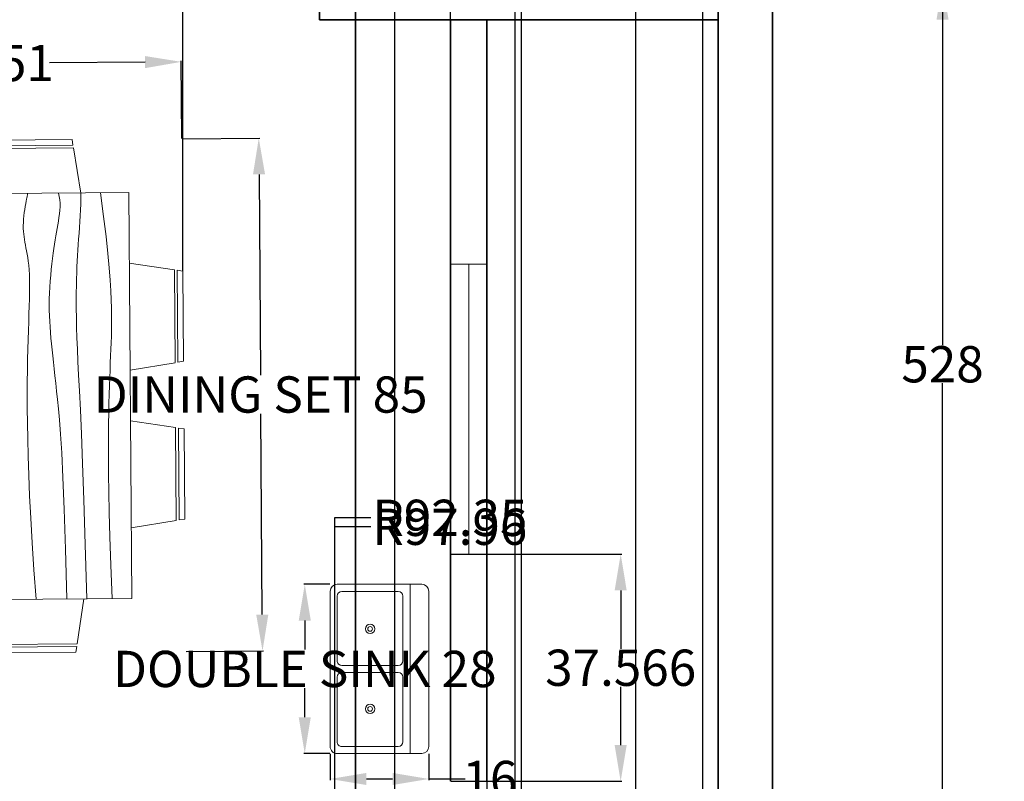
# Model space of a CAD drawing. Units: inches. Extents: x 351 to 774, y 111 to 703.
# Tile 4 of 6: x 608 to 771, y 338 to 464. Entities that reach past the tile are written whole.
import ezdxf

# ---------------------------------------------------------------- set-up
doc = ezdxf.new("R2010")
doc.units = ezdxf.units.IN
doc.header["$MEASUREMENT"] = 0
for name, color, linetype, lineweight in [('A-ANNO-DIMS', 2, 'Continuous', 18), ('A-FLOR-FIXT', 9, 'Continuous', 18), ('A-FURN', 8, 'Continuous', 18), ('A-GLAZ', 4, 'Continuous', 18), ('A-WALL', 7, 'Continuous', 35)]:
    doc.layers.add(name, color=color, linetype=linetype, lineweight=lineweight)
doc.styles.get("Standard").update_dxf_attribs({"font": 'arial.ttf'})
doc.dimstyles.get("Standard").update_dxf_attribs({"dimtxt": 6, "dimasz": 6, "dimexe": 0.18, "dimexo": 0.0625, "dimgap": 0.09, "dimtad": 0, "dimtih": 1, "dimtoh": 1, "dimdec": 0, "dimzin": 0, "dimdsep": 46, "dimlunit": 3, "dimtxsty": 'Standard', "dimcen": 0.09, "dimadec": 0, "dimazin": 0, "dimtfac": 1, "dimtdec": 0, "dimtofl": 0, "dimtmove": 0, "dimatfit": 3, "dimfxl": 1, "dimtolj": 1, "dimtzin": 0, "dimarcsym": 0})

# ---------------------------------------------------------------- blocks, each defined once
blk = doc.blocks.new('Dining Set - 36 x 72 in.')
for p, q in [((-22, 27.5), (-22.1562, 26.50042)), ((-5.8416, 26.5), (-22.1534, 26.5)), ((-22, 27.5), (-6, 27.5)), ((-5.8437, 26.49966), (-6, 27.5)), ((6, 27.5), (5.8438, 26.50042)), ((22.1584, 26.5), (5.8466, 26.5)), ((6, 27.5), (22, 27.5)), ((22.1563, 26.49966), (22, 27.5)), ((-22.2343, 26.00059), (-23.4847, 17.99762)), ((-22.2304, 26), (-5.7608, 26)), ((-4.5152, 17.99762), (-5.7655, 25.99926)), ((5.7657, 26.00059), (4.5153, 17.99762)), ((5.7696, 26), (22.2392, 26)), ((23.4848, 17.99762), (22.2345, 25.99926)), ((36, 18), (-36, 18)), ((-36, 18), (-36, -18)), ((36, -18), (36, 18)), ((-44.0006, 8.23428), (-35.9976, 9.48474)), ((44.0006, 8.23428), (35.9976, 9.48474)), ((-45.5, 8), (-44.5004, 8.15617)), ((-45.5, 8), (-45.5, -8)), ((-44.5, -8.15843), (-44.5, 8.15338)), ((-44, 8.23041), (-44, -8.23915)), ((44, 8.23041), (44, -8.23915)), ((44.5, -8.15843), (44.5, 8.15338)), ((45.5, 8), (44.5005, 8.15617)), ((45.5, 8), (45.5, -8)), ((-44.4997, -8.15631), (-45.5, -8)), ((-35.9976, -9.48476), (-43.9993, -8.2345)), ((35.9976, -9.48476), (43.9993, -8.2345)), ((44.4997, -8.15631), (45.5, -8)), ((-36, -18), (36, -18)), ((-22.2343, -26.0006), (-23.4847, -17.99762)), ((-4.5152, -17.99762), (-5.7655, -25.99928)), ((5.7657, -26.0006), (4.5153, -17.99762)), ((23.4848, -17.99762), (22.2345, -25.99928)), ((-22.2304, -26), (-5.7608, -26)), ((5.7696, -26), (22.2392, -26)), ((-22, -27.5), (-22.1562, -26.50044)), ((-5.8416, -26.5), (-22.1534, -26.5)), ((-22, -27.5), (-6, -27.5)), ((-5.8437, -26.49967), (-6, -27.5)), ((6, -27.5), (5.8438, -26.50044)), ((22.1584, -26.5), (5.8466, -26.5)), ((6, -27.5), (22, -27.5)), ((22.1563, -26.49967), (22, -27.5))]:
    blk.add_line(p, q)
for points in [[(-36, 15), (-31.1772, 14.97754), (-26.8079, 14.91406), (-22.8538, 14.81543), (-19.276, 14.6875), (-16.0362, 14.53613), (-13.0957, 14.36718), (-10.4159, 14.18652), (-7.9583, 14), (-5.6904, 13.81315), (-3.6035, 13.63021), (-1.6954, 13.45508), (0.0365, 13.29166), (1.5945, 13.14388), (2.9811, 13.01562), (4.1988, 12.9108), (5.25, 12.83333), (6.1393, 12.78613), (6.8802, 12.76823), (7.4883, 12.77767), (7.9792, 12.8125), (8.3685, 12.87077), (8.6719, 12.95052), (8.9049, 13.0498), (9.0833, 13.16666), (9.2205, 13.29899), (9.3216, 13.44401), (9.3895, 13.59879), (9.4271, 13.76041), (9.4373, 13.92594), (9.4232, 14.09245), (9.3875, 14.257), (9.3333, 14.41666), (9.2638, 14.56917), (9.1836, 14.71484), (9.0975, 14.85465), (9.0104, 14.98958), (8.9272, 15.1206), (8.8529, 15.2487), (8.7922, 15.37483), (8.75, 15.5), (8.7305, 15.62467), (8.7344, 15.74739), (8.7617, 15.86621), (8.8125, 15.97916), (8.8867, 16.08431), (8.9844, 16.17968), (9.1055, 16.26334), (9.25, 16.33333), (9.4189, 16.38802), (9.6172, 16.42708), (9.8506, 16.45052), (10.125, 16.45833), (10.4463, 16.45052), (10.8203, 16.42708), (11.2529, 16.38802), (11.75, 16.33333), (12.3184, 16.26318), (12.9694, 16.17838), (13.7151, 16.07991), (14.5677, 15.96875), (15.5395, 15.84586), (16.6426, 15.71224), (17.8893, 15.56884), (19.2917, 15.41666), (20.859, 15.25667), (22.5879, 15.08984), (24.4721, 14.91715), (26.5052, 14.73958), (28.6809, 14.5581), (30.9929, 14.3737), (33.4347, 14.18733), (36, 14)], [(-36, 10), (-28.9766, 10.14274), (-23.1725, 10.20442), (-18.4241, 10.19775), (-14.5677, 10.13541), (-11.4399, 10.03011), (-8.877, 9.89453), (-6.7154, 9.74137), (-4.7917, 9.58333), (-2.9698, 9.43082), (-1.2246, 9.28515), (0.4415, 9.14534), (2.026, 9.01041), (3.5266, 8.87939), (4.9408, 8.7513), (6.266, 8.62516), (7.5, 8.5), (8.6411, 8.37549), (9.6914, 8.2539), (10.6538, 8.13818), (11.5312, 8.03125), (12.3267, 7.93603), (13.043, 7.85547), (13.6831, 7.79248), (14.25, 7.75), (14.7471, 7.7303), (15.1797, 7.73307), (15.5537, 7.75732), (15.875, 7.80208), (16.1494, 7.86637), (16.3828, 7.94922), (16.5811, 8.04964), (16.75, 8.16666), (16.8944, 8.29915), (17.0143, 8.44531), (17.1089, 8.60319), (17.1771, 8.77083), (17.218, 8.94629), (17.2305, 9.1276), (17.2137, 9.31282), (17.1667, 9.5), (17.0895, 9.6875), (16.987, 9.875), (16.8649, 10.0625), (16.7292, 10.25), (16.5856, 10.4375), (16.4401, 10.625), (16.2985, 10.8125), (16.1667, 11), (16.05, 11.18733), (15.9518, 11.3737), (15.8752, 11.5581), (15.8229, 11.73958), (15.798, 11.91715), (15.8034, 12.08984), (15.842, 12.25667), (15.9167, 12.41666), (16.0295, 12.56836), (16.1784, 12.70833), (16.3605, 12.83268), (16.5729, 12.9375), (16.8127, 13.01888), (17.0768, 13.07291), (17.3625, 13.0957), (17.6667, 13.08333), (17.9894, 13.03312), (18.3418, 12.94726), (18.7382, 12.82918), (19.1927, 12.68229), (19.7195, 12.51001), (20.3327, 12.31575), (21.0465, 12.10294), (21.875, 11.875), (22.8357, 11.63354), (23.959, 11.37304), (25.2786, 11.08618), (26.8282, 10.76562), (28.6414, 10.40405), (30.752, 9.99414), (33.1936, 9.52856), (36, 9)], [(-36, 5.5), (-30.7157, 5.3348), (-26.069, 5.20963), (-21.9946, 5.11767), (-18.4271, 5.05208), (-15.3009, 5.00602), (-12.5508, 4.97265), (-10.1112, 4.94515), (-7.9167, 4.91666), (-5.909, 4.88167), (-4.0586, 4.83984), (-2.3429, 4.79215), (-0.7396, 4.73958), (0.7739, 4.6831), (2.22, 4.6237), (3.6213, 4.56233), (5, 4.5), (6.373, 4.43782), (7.7344, 4.3776), (9.0723, 4.32129), (10.375, 4.27083), (11.6309, 4.22819), (12.8281, 4.19531), (13.9551, 4.17415), (15, 4.16666), (15.954, 4.17448), (16.819, 4.19791), (17.6001, 4.23698), (18.3021, 4.29166), (18.9299, 4.36198), (19.4883, 4.44791), (19.9823, 4.54948), (20.4167, 4.66666), (20.7969, 4.79899), (21.1302, 4.94401), (21.4245, 5.09879), (21.6875, 5.26041), (21.9271, 5.42594), (22.1511, 5.59245), (22.3672, 5.757), (22.5834, 5.91666), (22.8065, 6.06868), (23.0404, 6.21093), (23.2879, 6.34147), (23.5521, 6.45833), (23.8358, 6.55957), (24.142, 6.64323), (24.4735, 6.70735), (24.8334, 6.75), (25.2235, 6.76969), (25.642, 6.76692), (26.0858, 6.74267), (26.5521, 6.69791), (27.0379, 6.63362), (27.5404, 6.55078), (28.0565, 6.45036), (28.5834, 6.33333), (29.1242, 6.19987), (29.7071, 6.04687), (30.3661, 5.87044), (31.1354, 5.66666), (32.0493, 5.43164), (33.142, 5.16146), (34.4475, 4.85221), (36, 4.5)], [(-36, -1), (-30.7915, -0.6591), (-26.0195, -0.38216), (-21.6519, -0.16284), (-17.6563, 0.00521), (-14.0005, 0.12833), (-10.6523, 0.21289), (-7.5796, 0.26522), (-4.75, 0.29166), (-2.134, 0.29793), (0.2878, 0.28711), (2.5317, 0.26163), (4.6146, 0.22396), (6.5529, 0.17651), (8.3633, 0.12174), (10.0623, 0.06209), (11.6667, 0), (13.1899, -0.06201), (14.6341, -0.1211), (15.9982, -0.17432), (17.2813, -0.21875), (18.4823, -0.25147), (19.6003, -0.26953), (20.6343, -0.27002), (21.5834, -0.25), (22.4481, -0.20768), (23.2357, -0.14584), (23.9549, -0.06836), (24.6146, 0.02083), (25.2235, 0.11784), (25.7904, 0.21875), (26.3241, 0.31966), (26.8334, 0.41666), (27.3265, 0.50618), (27.8099, 0.58593), (28.2894, 0.65397), (28.7709, 0.70833), (29.2601, 0.74707), (29.763, 0.76823), (30.2855, 0.76985), (30.8334, 0.75), (31.4088, 0.70784), (31.9994, 0.64713), (32.589, 0.57275), (33.1615, 0.48958), (33.7008, 0.4025), (34.1908, 0.3164), (34.6153, 0.23616), (34.9584, 0.16666), (35.2099, 0.11165), (35.3848, 0.07031), (35.504, 0.04069), (35.5886, 0.02083), (35.6594, 0.00879), (35.7377, 0.0026), (35.8442, 0.00032), (36, 0)], [(-36, -6.5), (-27.1843, -6.31267), (-20.084, -6.1263), (-14.469, -5.9419), (-10.1094, -5.76042), (-6.7752, -5.58285), (-4.2363, -5.41016), (-2.2629, -5.24333), (-0.625, -5.08334), (0.8708, -4.93099), (2.2715, -4.78646), (3.5872, -4.64974), (4.8281, -4.52084), (6.0046, -4.39974), (7.127, -4.28646), (8.2053, -4.18099), (9.25, -4.08334), (10.2705, -3.99382), (11.2734, -3.91407), (12.2647, -3.84603), (13.25, -3.79167), (14.2354, -3.75293), (15.2266, -3.73177), (16.2295, -3.73015), (17.25, -3.75), (18.2912, -3.79248), (19.3451, -3.85547), (20.4009, -3.93604), (21.4479, -4.03125), (22.4754, -4.13819), (23.4727, -4.25391), (24.4289, -4.37549), (25.3334, -4.5), (26.1785, -4.62492), (26.9694, -4.74935), (27.7145, -4.87281), (28.4219, -4.99479), (29.1, -5.11483), (29.7572, -5.23242), (30.4016, -5.34709), (31.0417, -5.45834), (31.6837, -5.56437), (32.3262, -5.65821), (32.9658, -5.73153), (33.599, -5.77604), (34.2224, -5.78345), (34.8327, -5.74545), (35.4264, -5.65373), (36, -5.5)], [(-36, -10), (-26.4022, -9.81299), (-18.4675, -9.62891), (-11.9839, -9.45069), (-6.7396, -9.28125), (-2.5226, -9.12354), (0.8789, -8.98047), (3.6769, -8.85498), (6.0833, -8.75), (8.2767, -8.66765), (10.3021, -8.60677), (12.1712, -8.56543), (13.8958, -8.54167), (15.4876, -8.53353), (16.9583, -8.53907), (18.3197, -8.55632), (19.5834, -8.58334), (20.7616, -8.61841), (21.8685, -8.66081), (22.9188, -8.71004), (23.9271, -8.76563), (24.9081, -8.82707), (25.8763, -8.89388), (26.8465, -8.96558), (27.8334, -9.04167), (28.8474, -9.12118), (29.8828, -9.20117), (30.93, -9.27824), (31.9792, -9.34896), (33.0205, -9.40991), (34.0443, -9.45768), (35.0407, -9.48885), (36, -9.5)], [(-36, -14.5), (-30.0881, -14.33513), (-25.0332, -14.21224), (-20.7312, -14.12647), (-17.0781, -14.07292), (-13.97, -14.04671), (-11.3027, -14.04297), (-8.9724, -14.05681), (-6.875, -14.08334), (-4.9224, -14.11833), (-3.0905, -14.16016), (-1.3709, -14.20785), (0.2448, -14.26042), (1.7647, -14.3169), (3.1973, -14.3763), (4.5507, -14.43767), (5.8333, -14.5), (7.0554, -14.5621), (8.235, -14.62175), (9.3922, -14.67652), (10.5469, -14.72396), (11.7192, -14.76164), (12.929, -14.78711), (14.1965, -14.79794), (15.5417, -14.79167), (16.9933, -14.76424), (18.6152, -14.70508), (20.4804, -14.60197), (22.6615, -14.44271), (25.2312, -14.21509), (28.2624, -13.9069), (31.8277, -13.50594), (36, -13)]]:
    blk.add_lwpolyline(points)
blk = doc.blocks.new('Sink-double - 36 in top')
for p, q in [((-18, -4), (18, -4)), ((-0.75, -18.5), (-0.75, -6.5)), ((0.75, -6.5), (0.75, -18.5))]:
    blk.add_line(p, q)
for points in [[(-16.5, 0), (16.5, 0)], [(-18, -19.5), (-18, -1.5)], [(18, -1.5), (18, -19.5)], [(-15.5, -5.5), (-1.75, -5.5)], [(1.75, -5.5), (15.5, -5.5)], [(-16.5, -18.5), (-16.5, -6.5)], [(16.5, -6.5), (16.5, -18.5)], [(-1.75, -19.5), (-15.5, -19.5)], [(15.5, -19.5), (1.75, -19.5)], [(16.5, -21), (-16.5, -21)]]:
    blk.add_lwpolyline(points)
for centre, radius in [((-8.5, -12.5), 1), ((-8.5, -12.5), 0.5), ((8.5, -12.5), 1), ((8.5, -12.5), 0.5)]:
    blk.add_circle(centre, radius)
for centre, radius, start, end in [((-16.5, -1.5), 1.5, 90, 180), ((16.5, -1.5), 1.5, 0, 90), ((-15.5, -6.5), 1, 90, 180), ((-1.75, -6.5), 1, 0, 90), ((1.75, -6.5), 1, 90, 180), ((15.5, -6.5), 1, 0, 90), ((-15.5, -18.5), 1, 180, 270), ((-1.75, -18.5), 1, 270, 0), ((1.75, -18.5), 1, 180, 270), ((15.5, -18.5), 1, 270, 0), ((-16.5, -19.5), 1.5, 180, 270), ((16.5, -19.5), 1.5, 270, 0)]:
    blk.add_arc(centre, radius, start, end)
blk = doc.blocks.new('WIN-48IN-6IN-WALL')
blk.add_line((3, 48), (3, 0))
blk.add_lwpolyline([(0, 48), (6, 48), (6, 0), (0, 0)], close=True)
blk = doc.blocks.new('*D32')
at = {"layer": 'A-ANNO-DIMS', "color": 0, "lineweight": -2, "transparency": 16777216}
for p, q in [((696.79, 480.27), (696.79, 476.4)), ((721.84, 480.27), (721.84, 476.4)), ((702.79, 476.58), (715.84, 476.58)), ((721.84, 476.58), (727.84, 476.58))]:
    blk.add_line(p, q, dxfattribs=at)
at = {"layer": 'A-ANNO-DIMS', "color": 0, "transparency": 16777216}
for points in [[(702.79, 477.58), (702.79, 475.58), (696.79, 476.58)], [(715.84, 477.58), (715.84, 475.58), (721.84, 476.58)]]:
    blk.add_solid(points, dxfattribs=at)
at = {"layer": 'Defpoints', "color": 0, "transparency": 16777216}
for p in [(696.79, 480.33), (721.84, 480.33), (721.84, 476.58)]:
    blk.add_point(p, dxfattribs=at)
at = {"layer": 'A-ANNO-DIMS', "color": 0, "transparency": 16777216, "insert": (750.8, 476.58), "char_height": 6, "attachment_point": 5}
blk.add_mtext('\\A1;WC 25 TYP.', dxfattribs=at)
blk = doc.blocks.new('*D36')
at = {"layer": 'A-ANNO-DIMS', "color": 0, "lineweight": -2, "transparency": 16777216}
for p, q in [((635.35, 444.55), (648.2, 444.64)), ((648.06, 438.64), (648.31, 405.42)), ((648.6, 365.81), (648.35, 399.03)), ((635.98, 359.72), (648.82, 359.81))]:
    blk.add_line(p, q, dxfattribs=at)
at = {"layer": 'A-ANNO-DIMS', "color": 0, "transparency": 16777216}
for points in [[(649.06, 438.65), (647.06, 438.64), (648.02, 444.64)], [(649.6, 365.82), (647.6, 365.8), (648.64, 359.81)]]:
    blk.add_solid(points, dxfattribs=at)
at = {"layer": 'Defpoints', "color": 0, "transparency": 16777216}
for p in [(635.29, 444.55), (648.02, 444.64), (635.92, 359.72)]:
    blk.add_point(p, dxfattribs=at)
at = {"layer": 'A-ANNO-DIMS', "color": 0, "transparency": 16777216, "insert": (648.33, 402.23), "char_height": 6, "attachment_point": 5}
blk.add_mtext('\\A1;DINING SET 85', dxfattribs=at)
blk = doc.blocks.new('*D37')
at = {"layer": 'A-ANNO-DIMS', "color": 0, "lineweight": -2, "transparency": 16777216}
for p, q in [((584.02, 444.23), (583.93, 457.08)), ((589.93, 456.94), (605.75, 457.06)), ((629.2, 457.23), (613.37, 457.11)), ((635.29, 444.61), (635.2, 457.45))]:
    blk.add_line(p, q, dxfattribs=at)
at = {"layer": 'A-ANNO-DIMS', "color": 0, "transparency": 16777216}
for points in [[(629.19, 458.23), (629.21, 456.23), (635.2, 457.27)], [(589.92, 457.94), (589.93, 455.94), (583.93, 456.9)]]:
    blk.add_solid(points, dxfattribs=at)
at = {"layer": 'Defpoints', "color": 0, "transparency": 16777216}
for p in [(583.93, 456.9), (584.02, 444.17), (635.29, 444.55)]:
    blk.add_point(p, dxfattribs=at)
at = {"layer": 'A-ANNO-DIMS', "color": 0, "transparency": 16777216, "insert": (609.56, 457.08), "char_height": 6, "attachment_point": 5}
blk.add_mtext('\\A1;51', dxfattribs=at)
blk = doc.blocks.new('*D38')
at = {"layer": 'A-ANNO-DIMS', "color": 0, "lineweight": -2, "transparency": 16777216}
for p, q in [((659.77, 370.83), (655.45, 370.83)), ((655.63, 364.83), (655.63, 360.03)), ((655.63, 348.83), (655.63, 353.64)), ((659.77, 342.83), (655.45, 342.83))]:
    blk.add_line(p, q, dxfattribs=at)
at = {"layer": 'A-ANNO-DIMS', "color": 0, "transparency": 16777216}
for points in [[(654.63, 364.83), (656.63, 364.83), (655.63, 370.83)], [(654.63, 348.83), (656.63, 348.83), (655.63, 342.83)]]:
    blk.add_solid(points, dxfattribs=at)
at = {"layer": 'Defpoints', "color": 0, "transparency": 16777216}
for p in [(659.83, 370.83), (655.63, 342.83), (659.83, 342.83)]:
    blk.add_point(p, dxfattribs=at)
at = {"layer": 'A-ANNO-DIMS', "color": 0, "transparency": 16777216, "insert": (655.63, 356.83), "char_height": 6, "attachment_point": 5}
blk.add_mtext('\\A1;DOUBLE SINK 28', dxfattribs=at)
blk = doc.blocks.new('*D39')
at = {"layer": 'A-ANNO-DIMS', "color": 0, "lineweight": -2, "transparency": 16777216}
for p, q in [((659.83, 342.77), (659.83, 338.45)), ((676.17, 342.77), (676.17, 338.45)), ((665.83, 338.63), (670.17, 338.63)), ((676.17, 338.63), (682.17, 338.63))]:
    blk.add_line(p, q, dxfattribs=at)
at = {"layer": 'A-ANNO-DIMS', "color": 0, "transparency": 16777216}
for points in [[(665.83, 339.63), (665.83, 337.63), (659.83, 338.63)], [(670.17, 339.63), (670.17, 337.63), (676.17, 338.63)]]:
    blk.add_solid(points, dxfattribs=at)
at = {"layer": 'Defpoints', "color": 0, "transparency": 16777216}
for p in [(659.83, 342.83), (676.17, 342.83), (676.17, 338.63)]:
    blk.add_point(p, dxfattribs=at)
at = {"layer": 'A-ANNO-DIMS', "color": 0, "transparency": 16777216, "insert": (686.27, 338.63), "char_height": 6, "attachment_point": 5}
blk.add_mtext('\\A1;16', dxfattribs=at)
blk = doc.blocks.new('*D47')
at = {"layer": 'A-ANNO-DIMS', "color": 0, "lineweight": -2, "transparency": 16777216}
for p, q in [((733.11, 671.24), (761.37, 671.24)), ((761.19, 665.24), (761.19, 410.4)), ((761.19, 149.24), (761.19, 404.09)), ((733.11, 143.24), (761.37, 143.24))]:
    blk.add_line(p, q, dxfattribs=at)
at = {"layer": 'A-ANNO-DIMS', "color": 0, "transparency": 16777216}
for points in [[(760.19, 665.24), (762.19, 665.24), (761.19, 671.24)], [(760.19, 149.24), (762.19, 149.24), (761.19, 143.24)]]:
    blk.add_solid(points, dxfattribs=at)
at = {"layer": 'Defpoints', "color": 0, "transparency": 16777216}
for p in [(733.04, 671.24), (761.19, 671.24), (733.04, 143.24)]:
    blk.add_point(p, dxfattribs=at)
at = {"layer": 'A-ANNO-DIMS', "color": 0, "transparency": 16777216, "insert": (761.19, 407.24), "char_height": 6, "attachment_point": 5}
blk.add_mtext('\\A1;528', dxfattribs=at)
blk = doc.blocks.new('*D68')
at = {"layer": 'A-ANNO-DIMS', "color": 0, "lineweight": -2, "transparency": 16777216}
for p, q in [((685.77, 338.18), (685.77, 114.91)), ((724.04, 338.18), (724.04, 114.91)), ((691.77, 115.09), (694.69, 115.09)), ((718.04, 115.09), (715.12, 115.09))]:
    blk.add_line(p, q, dxfattribs=at)
at = {"layer": 'A-ANNO-DIMS', "color": 0, "transparency": 16777216}
for points in [[(691.77, 116.09), (691.77, 114.09), (685.77, 115.09)], [(718.04, 116.09), (718.04, 114.09), (724.04, 115.09)]]:
    blk.add_solid(points, dxfattribs=at)
at = {"layer": 'Defpoints', "color": 0, "transparency": 16777216}
for p in [(685.77, 338.24), (724.04, 338.24), (724.04, 115.09)]:
    blk.add_point(p, dxfattribs=at)
at = {"layer": 'A-ANNO-DIMS', "color": 0, "transparency": 16777216, "insert": (704.9, 115.09), "char_height": 6, "attachment_point": 5}
blk.add_mtext('\\A1;38.28', dxfattribs=at)
blk = doc.blocks.new('*D69')
at = {"layer": 'A-ANNO-DIMS', "color": 0, "lineweight": -2, "transparency": 16777216}
for p, q in [((724.04, 473.44), (724.04, 114.91)), ((664.04, 470.18), (664.04, 114.91)), ((670.04, 115.09), (689.65, 115.09)), ((718.04, 115.09), (698.44, 115.09))]:
    blk.add_line(p, q, dxfattribs=at)
at = {"layer": 'A-ANNO-DIMS', "color": 0, "transparency": 16777216}
for points in [[(670.04, 116.09), (670.04, 114.09), (664.04, 115.09)], [(718.04, 116.09), (718.04, 114.09), (724.04, 115.09)]]:
    blk.add_solid(points, dxfattribs=at)
at = {"layer": 'Defpoints', "color": 0, "transparency": 16777216}
for p in [(724.04, 473.5), (664.04, 470.24), (724.04, 115.09)]:
    blk.add_point(p, dxfattribs=at)
at = {"layer": 'A-ANNO-DIMS', "color": 0, "transparency": 16777216, "insert": (694.04, 115.09), "char_height": 6, "attachment_point": 5}
blk.add_mtext('\\A1;60', dxfattribs=at)
blk = doc.blocks.new('*D81')
at = {"layer": 'A-ANNO-DIMS', "color": 0, "lineweight": -2, "transparency": 16777216}
for p, q in [((679.83, 375.81), (708.1, 375.81)), ((707.92, 369.81), (707.92, 360.18)), ((707.92, 344.24), (707.92, 353.87)), ((679.83, 338.24), (708.1, 338.24))]:
    blk.add_line(p, q, dxfattribs=at)
at = {"layer": 'A-ANNO-DIMS', "color": 0, "transparency": 16777216}
for points in [[(706.92, 369.81), (708.92, 369.81), (707.92, 375.81)], [(706.92, 344.24), (708.92, 344.24), (707.92, 338.24)]]:
    blk.add_solid(points, dxfattribs=at)
at = {"layer": 'Defpoints', "color": 0, "transparency": 16777216}
for p in [(679.77, 375.81), (679.77, 338.24), (707.92, 338.24)]:
    blk.add_point(p, dxfattribs=at)
at = {"layer": 'A-ANNO-DIMS', "color": 0, "transparency": 16777216, "insert": (707.92, 357.03), "char_height": 6, "attachment_point": 5}
blk.add_mtext('\\A1;37.566', dxfattribs=at)
blk = doc.blocks.new('*D86')
at = {"layer": 'A-ANNO-DIMS', "color": 0, "lineweight": -2, "transparency": 16777216}
for p, q in [((710.41, 152.3), (710.41, 699.57)), ((716.41, 699.39), (718.04, 699.39)), ((724.04, 152.3), (724.04, 699.57)), ((724.04, 699.39), (730.04, 699.39))]:
    blk.add_line(p, q, dxfattribs=at)
at = {"layer": 'A-ANNO-DIMS', "color": 0, "transparency": 16777216}
for points in [[(716.41, 700.39), (716.41, 698.39), (710.41, 699.39)], [(718.04, 700.39), (718.04, 698.39), (724.04, 699.39)]]:
    blk.add_solid(points, dxfattribs=at)
at = {"layer": 'Defpoints', "color": 0, "transparency": 16777216}
for p in [(724.04, 699.39), (710.41, 152.24), (724.04, 152.24)]:
    blk.add_point(p, dxfattribs=at)
at = {"layer": 'A-ANNO-DIMS', "color": 0, "transparency": 16777216, "insert": (742.3, 699.39), "char_height": 6, "attachment_point": 5}
blk.add_mtext('\\A1;13.633', dxfattribs=at)
blk = doc.blocks.new('*D87')
at = {"layer": 'A-ANNO-DIMS', "color": 0, "lineweight": -2, "transparency": 16777216}
for p, q in [((691.51, 206.3), (691.51, 699.57)), ((697.51, 699.39), (702.14, 699.39)), ((715.51, 699.39), (710.89, 699.39)), ((721.51, 206.3), (721.51, 699.57))]:
    blk.add_line(p, q, dxfattribs=at)
at = {"layer": 'A-ANNO-DIMS', "color": 0, "transparency": 16777216}
for points in [[(697.51, 700.39), (697.51, 698.39), (691.51, 699.39)], [(715.51, 700.39), (715.51, 698.39), (721.51, 699.39)]]:
    blk.add_solid(points, dxfattribs=at)
at = {"layer": 'Defpoints', "color": 0, "transparency": 16777216}
for p in [(721.51, 699.39), (691.51, 206.24), (721.51, 206.24)]:
    blk.add_point(p, dxfattribs=at)
at = {"layer": 'A-ANNO-DIMS', "color": 0, "transparency": 16777216, "insert": (706.51, 699.39), "char_height": 6, "attachment_point": 5}
blk.add_mtext('\\A1;30', dxfattribs=at)
blk = doc.blocks.new('*D88')
at = {"layer": 'A-ANNO-DIMS', "color": 0, "lineweight": -2, "transparency": 16777216}
for p, q in [((658.043027, 699.392076), (652.043027, 699.392076)), ((664.043027, 200.304576), (664.043027, 699.572076)), ((691.510725, 200.304576), (691.510725, 699.572076)), ((697.510725, 699.392076), (703.510725, 699.392076))]:
    blk.add_line(p, q, dxfattribs=at)
at = {"layer": 'A-ANNO-DIMS', "color": 0, "transparency": 16777216}
for points in [[(658.043027, 700.392076), (658.043027, 698.392076), (664.043027, 699.392076)], [(697.510725, 700.392076), (697.510725, 698.392076), (691.510725, 699.392076)]]:
    blk.add_solid(points, dxfattribs=at)
at = {"layer": 'Defpoints', "color": 0, "transparency": 16777216}
for p in [(691.510725, 699.392076), (664.043027, 200.242076), (691.510725, 200.242076)]:
    blk.add_point(p, dxfattribs=at)
at = {"layer": 'A-ANNO-DIMS', "color": 0, "transparency": 16777216, "insert": (677.776876, 699.392076), "char_height": 6, "attachment_point": 5}
blk.add_mtext('\\A1;27.47', dxfattribs=at)
blk = doc.blocks.new('*D96')
at = {"layer": 'A-ANNO-DIMS', "color": 0, "lineweight": -2, "transparency": 16777216}
for p, q in [((635.45, 422.7), (635.45, 699.57)), ((641.45, 699.39), (647.85, 699.39)), ((673.77, 699.39), (667.36, 699.39)), ((679.77, 423.87), (679.77, 699.57))]:
    blk.add_line(p, q, dxfattribs=at)
at = {"layer": 'A-ANNO-DIMS', "color": 0, "transparency": 16777216}
for points in [[(641.45, 700.39), (641.45, 698.39), (635.45, 699.39)], [(673.77, 700.39), (673.77, 698.39), (679.77, 699.39)]]:
    blk.add_solid(points, dxfattribs=at)
at = {"layer": 'Defpoints', "color": 0, "transparency": 16777216}
for p in [(679.77, 699.39), (679.77, 423.81), (635.45, 422.64)]:
    blk.add_point(p, dxfattribs=at)
at = {"layer": 'A-ANNO-DIMS', "color": 0, "transparency": 16777216, "insert": (657.61, 699.39), "char_height": 6, "attachment_point": 5}
blk.add_mtext('\\A1;44.31', dxfattribs=at)
blk = doc.blocks.new('*D101')
at = {"layer": 'A-ANNO-DIMS', "color": 0, "lineweight": -2, "transparency": 16777216}
for p, q in [((658.04, 699.39), (652.04, 699.39)), ((664.04, 152.3), (664.04, 699.57)), ((690.48, 153.55), (690.48, 699.57)), ((696.48, 699.39), (702.48, 699.39))]:
    blk.add_line(p, q, dxfattribs=at)
at = {"layer": 'A-ANNO-DIMS', "color": 0, "transparency": 16777216}
for points in [[(658.04, 700.39), (658.04, 698.39), (664.04, 699.39)], [(696.48, 700.39), (696.48, 698.39), (690.48, 699.39)]]:
    blk.add_solid(points, dxfattribs=at)
at = {"layer": 'Defpoints', "color": 0, "transparency": 16777216}
for p in [(664.04, 699.39), (690.48, 153.49), (664.04, 152.24)]:
    blk.add_point(p, dxfattribs=at)
at = {"layer": 'A-ANNO-DIMS', "color": 0, "transparency": 16777216, "insert": (677.26, 699.39), "char_height": 6, "attachment_point": 5}
blk.add_mtext('\\A1;26.433', dxfattribs=at)
blk = doc.blocks.new('*D103')
at = {"layer": 'A-ANNO-DIMS', "color": 0, "lineweight": -2, "transparency": 16777216}
for p, q in [((761.19, 486.33), (761.19, 492.33)), ((721.9, 480.33), (761.37, 480.33)), ((724.11, 470.24), (761.37, 470.24)), ((761.19, 464.24), (761.19, 458.24))]:
    blk.add_line(p, q, dxfattribs=at)
at = {"layer": 'A-ANNO-DIMS', "color": 0, "transparency": 16777216}
for points in [[(760.19, 486.33), (762.19, 486.33), (761.19, 480.33)], [(760.19, 464.24), (762.19, 464.24), (761.19, 470.24)]]:
    blk.add_solid(points, dxfattribs=at)
at = {"layer": 'Defpoints', "color": 0, "transparency": 16777216}
for p in [(721.84, 480.33), (724.04, 470.24), (761.19, 470.24)]:
    blk.add_point(p, dxfattribs=at)
at = {"layer": 'A-ANNO-DIMS', "color": 0, "transparency": 16777216, "insert": (761.19, 475.29), "char_height": 6, "attachment_point": 5}
blk.add_mtext('\\A1;10.09', dxfattribs=at)
blk = doc.blocks.new('*D108')
at = {"layer": 'A-ANNO-DIMS', "color": 0, "lineweight": -2, "transparency": 16777216}
for p, q in [((664.04, 527.44), (664.04, 114.91)), ((670.51, 515.76), (670.51, 114.91)), ((658.04, 115.09), (652.04, 115.09)), ((676.51, 115.09), (682.51, 115.09))]:
    blk.add_line(p, q, dxfattribs=at)
at = {"layer": 'A-ANNO-DIMS', "color": 0, "transparency": 16777216}
for points in [[(658.04, 116.09), (658.04, 114.09), (664.04, 115.09)], [(676.51, 116.09), (676.51, 114.09), (670.51, 115.09)]]:
    blk.add_solid(points, dxfattribs=at)
at = {"layer": 'Defpoints', "color": 0, "transparency": 16777216}
for p in [(664.04, 527.5), (670.51, 515.82), (664.04, 115.09)]:
    blk.add_point(p, dxfattribs=at)
at = {"layer": 'A-ANNO-DIMS', "color": 0, "transparency": 16777216, "insert": (641.84, 115.09), "char_height": 6, "attachment_point": 5}
blk.add_mtext('\\A1;6.472', dxfattribs=at)
blk = doc.blocks.new('*D110')
at = {"layer": 'A-ANNO-DIMS', "color": 0, "lineweight": -2, "transparency": 16777216}
for p, q in [((666.56, 380.35), (660.56, 380.35)), ((660.56, 380.35), (660.56, 327.58)), ((660.47, 223.61), (660.65, 223.61)), ((660.56, 223.52), (660.56, 223.7))]:
    blk.add_line(p, q, dxfattribs=at)
at = {"layer": 'A-ANNO-DIMS', "color": 0, "transparency": 16777216}
blk.add_solid([(659.56, 327.58), (661.56, 327.58), (660.56, 321.58)], dxfattribs=at)
at = {"layer": 'Defpoints', "color": 0, "transparency": 16777216}
for p in [(660.56, 321.58), (660.56, 223.61)]:
    blk.add_point(p, dxfattribs=at)
at = {"layer": 'A-ANNO-DIMS', "color": 0, "transparency": 16777216, "insert": (679.64, 380.35), "char_height": 6, "attachment_point": 5}
blk.add_mtext('\\A1;R97.96', dxfattribs=at)
blk = doc.blocks.new('*D111')
at = {"layer": 'A-ANNO-DIMS', "color": 0, "lineweight": -2, "transparency": 16777216}
for p, q in [((666.56, 381.83), (660.56, 381.83)), ((660.56, 381.83), (660.56, 332.43)), ((660.47, 234.08), (660.65, 234.08)), ((660.56, 233.99), (660.56, 234.17))]:
    blk.add_line(p, q, dxfattribs=at)
at = {"layer": 'A-ANNO-DIMS', "color": 0, "transparency": 16777216}
blk.add_solid([(659.56, 332.43), (661.56, 332.43), (660.56, 326.43)], dxfattribs=at)
at = {"layer": 'Defpoints', "color": 0, "transparency": 16777216}
for p in [(660.56, 326.43), (660.56, 234.08)]:
    blk.add_point(p, dxfattribs=at)
at = {"layer": 'A-ANNO-DIMS', "color": 0, "transparency": 16777216, "insert": (679.66, 381.83), "char_height": 6, "attachment_point": 5}
blk.add_mtext('\\A1;R92.35', dxfattribs=at)

msp = doc.modelspace()

# ---------------------------------------------------------------- linework, layer by layer
at = {"layer": 'A-WALL'}
for p, q in [((658.043, 470.2421), (658.043, 464.2421)), ((658.043, 464.2421), (724.043, 464.2421)), ((679.7664, 464.2421), (679.7664, 338.2421)), ((685.7664, 464.2421), (685.7664, 338.2421)), ((724.043, 464.2421), (724.043, 338.2421))]:
    msp.add_line(p, q, dxfattribs=at)
msp.add_lwpolyline([(436.7781, 143.2421), (421.043, 143.2421), (421.043, 671.2421), (733.043, 671.2421), (733.043, 143.2421), (562.043, 143.2421)], dxfattribs=at)

# ---------------------------------------------------------------- block references
at = {"layer": 'A-FLOR-FIXT', "xscale": 0.7777777777777778, "yscale": 0.7777777777777778, "zscale": 0.7777777777777778, "rotation": 270}
msp.add_blockref('Sink-double - 36 in top', (676.1667, 356.8333), dxfattribs=at)
at = {"layer": 'A-FURN', "xscale": 0.9322251862135446, "yscale": 0.9322251862135446, "zscale": 0.9322251862135446, "rotation": 90.42208138352696}
msp.add_blockref('Dining Set - 36 x 72 in.', (609.9687, 401.9447), dxfattribs=at)
at = {"layer": 'A-GLAZ'}
msp.add_blockref('WIN-48IN-6IN-WALL', (679.7664, 375.8083), dxfattribs=at)

# ---------------------------------------------------------------- dimensions: what is measured, and where the dimension line sits
at = {"layer": 'A-ANNO-DIMS'}
for base, p1, p2, override, picture, middle in [((679.7664, 699.3921), (635.4531, 422.6419), (679.7664, 423.8083), {"dimdec": 2, "dimlfac": 1, "dimrnd": 0, "dimzin": 0, "dimdsep": 46, "dimlunit": 2}, '*D96', (657.6098, 699.3921)), ((691.5107, 699.3921), (664.043, 200.2421), (691.5107, 200.2421), {"dimdec": 2, "dimlfac": 1, "dimrnd": 0, "dimzin": 0, "dimdsep": 46, "dimlunit": 2}, '*D88', (677.7769, 699.3921)), ((664.043, 699.3921), (690.4757, 153.4918), (664.043, 152.2421), {"dimdec": 3, "dimlfac": 1, "dimrnd": 0, "dimzin": 0, "dimdsep": 46, "dimlunit": 2}, '*D101', (677.2594, 699.3921)), ((721.5107, 699.3921), (691.5107, 206.2421), (721.5107, 206.2421), {"dimdec": 0, "dimlfac": 1, "dimrnd": 0, "dimzin": 0, "dimdsep": 46, "dimlunit": 2}, '*D87', (706.5107, 699.3921)), ((724.043, 699.3921), (710.4102, 152.2421), (724.043, 152.2421), {"dimdec": 3, "dimlfac": 1, "dimrnd": 0, "dimzin": 0, "dimdsep": 46, "dimlunit": 2}, '*D86', (742.3049, 699.3921)), ((664.043, 115.0921), (670.5147, 515.8184), (664.043, 527.5), {"dimdec": 3, "dimlfac": 1, "dimrnd": 0, "dimzin": 0, "dimdsep": 46, "dimlunit": 2}, '*D108', (641.8439, 115.0921)), ((724.043, 115.0921), (664.043, 470.2421), (724.043, 473.5), {"dimdec": 0, "dimlfac": 1, "dimrnd": 0, "dimzin": 0, "dimdsep": 46, "dimlunit": 2}, '*D69', (694.043, 115.0921)), ((676.1667, 338.6333), (659.8333, 342.8333), (676.1667, 342.8333), {"dimdec": 0, "dimlfac": 1, "dimrnd": 0, "dimzin": 0, "dimdsep": 46, "dimlunit": 2}, '*D39', (686.2696, 338.6333)), ((724.043, 115.0921), (685.7664, 338.2421), (724.043, 338.2421), {"dimdec": 2, "dimlfac": 1, "dimrnd": 0, "dimzin": 0, "dimdsep": 46, "dimlunit": 2}, '*D68', (704.9047, 115.0921))]:
    dim = msp.add_linear_dim(base=base, p1=p1, p2=p2, dimstyle='Standard', override=override, dxfattribs=at)
    dim.commit()
    dim.dimension.update_dxf_attribs({"geometry": picture, "text_midpoint": middle})
for base, p1, p2, angle, override, picture, middle in [((761.193, 671.2421), (733.043, 143.2421), (733.043, 671.2421), 90, {"dimdec": 0, "dimlfac": 1, "dimrnd": 0, "dimzin": 0, "dimdsep": 46, "dimlunit": 2}, '*D47', (761.193, 407.2421)), ((761.193, 470.2421), (721.8351, 480.3324), (724.043, 470.2421), 90, {"dimdec": 2, "dimlfac": 1, "dimrnd": 0, "dimzin": 0, "dimdsep": 46, "dimlunit": 2}, '*D103', (761.193, 475.2873)), ((583.927, 456.8954), (635.2917, 444.5486), (584.0207, 444.1709), 180.422081, {"dimdec": 0, "dimlfac": 1, "dimrnd": 0, "dimzin": 0, "dimdsep": 46, "dimlunit": 2}, '*D37', (609.5625, 457.0843)), ((707.9164, 338.2421), (679.7664, 375.8083), (679.7664, 338.2421), 270, {"dimdec": 3, "dimlfac": 1, "dimrnd": 0, "dimzin": 0, "dimdsep": 46, "dimlunit": 2}, '*D81', (707.9164, 357.0252))]:
    dim = msp.add_linear_dim(base=base, p1=p1, p2=p2, angle=angle, dimstyle='Standard', override=override, dxfattribs=at)
    dim.commit()
    dim.dimension.update_dxf_attribs({"geometry": picture, "text_midpoint": middle})
dim = msp.add_linear_dim(base=(721.8351, 476.5764), p1=(696.7947, 480.3324), p2=(721.8351, 480.3324), text='WC <> TYP.', dimstyle='Standard', override={"dimdec": 0, "dimlfac": 1, "dimrnd": 0, "dimzin": 0, "dimdsep": 46, "dimlunit": 2}, dxfattribs=at)
dim.commit()
dim.dimension.update_dxf_attribs({"geometry": '*D32', "text_midpoint": (750.7976, 476.5764)})
for base, p1, p2, angle, text, picture, middle in [((648.0162, 444.6424), (635.9166, 359.7184), (635.2917, 444.5486), 90.422081, 'DINING SET <>', '*D36', (648.3287, 402.2273)), ((655.6333, 342.8333), (659.8333, 370.8333), (659.8333, 342.8333), 270, 'DOUBLE SINK <>', '*D38', (655.6333, 356.8333))]:
    dim = msp.add_linear_dim(base=base, p1=p1, p2=p2, angle=angle, text=text, dimstyle='Standard', override={"dimdec": 0, "dimlfac": 1, "dimrnd": 0, "dimzin": 0, "dimdsep": 46, "dimlunit": 2}, dxfattribs=at)
    dim.commit()
    dim.dimension.update_dxf_attribs({"geometry": picture, "text_midpoint": middle})
for center, mpoint, picture, middle in [((660.5567, 234.0791), (660.557, 326.4263), '*D111', (679.6642, 381.8345)), ((660.5567, 223.6144), (660.557, 321.5765), '*D110', (679.6397, 380.3538))]:
    dim = msp.add_radius_dim(center=center, mpoint=mpoint, dimstyle='Standard', override={"dimdec": 2, "dimlfac": 1, "dimrnd": 0, "dimzin": 0, "dimdsep": 46, "dimlunit": 2}, dxfattribs=at)
    dim.commit()
    dim.dimension.update_dxf_attribs({"geometry": picture, "text_midpoint": middle, "dimtype": 164})

doc.saveas('drawing.dxf')
